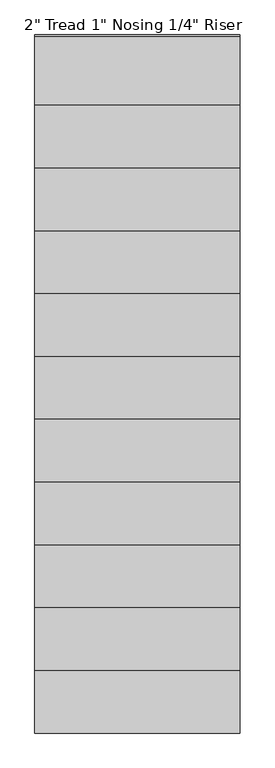
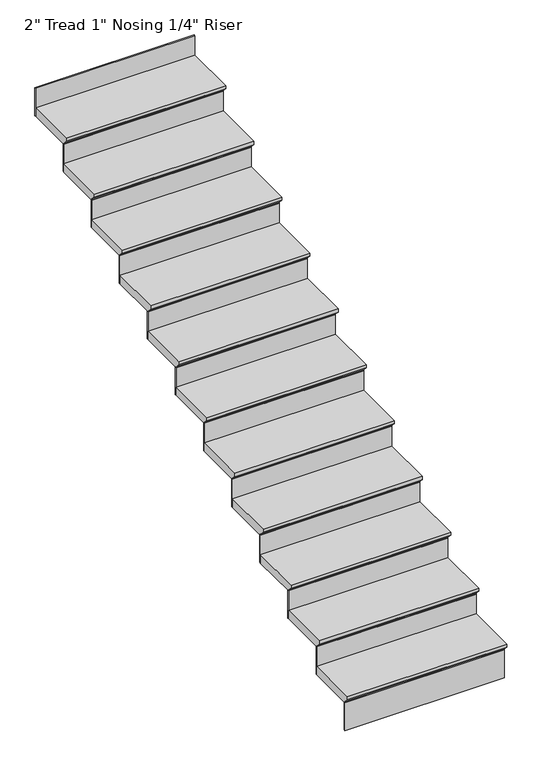
"""IFC4 building model written with IfcOpenShell, lengths in millimetres: stair flight geometry."""

from ifc_helpers import new_model, si_unit, frame, origin, place, context, project, spatial, polyline, outline, extrude, source, transform, mapped, element, save


def stair_flight_b0062ef7(model_context):
    return source(origin(), model_context, "Body", "SweptSolid", [
        extrude(outline(polyline([(-11795.059218, 4233.3333333), (-11490.259218, 4233.3333333), (-11490.259218, 4182.5333333), (-11769.659218, 4182.5333333), (-11769.659218, 4188.8833333), (-11795.059218, 4214.2833333), (-11795.059218, 4233.3333333)])), frame((-1903.2563134, 0.0, 0.0), z_axis=(1.0, 0.0, 0.0), x_axis=(0.0, 1.0, 0.0)), (0.0, 0.0, 1.0), 914.4),
        extrude(outline(polyline([(-988.8563134, -11763.309218), (-988.8563134, -11769.659218), (-1903.2563134, -11769.659218), (-1903.2563134, -11763.309218), (-988.8563134, -11763.309218)])), frame((0.0, 0.0, 4013.2), z_axis=(0.0, 0.0, 1.0), x_axis=(1.0, 0.0, 0.0)), (0.0, 0.0, 1.0), 169.3333333),
        extrude(outline(polyline([(-988.8563134, -11483.909218), (-988.8563134, -11490.259218), (-1903.2563134, -11490.259218), (-1903.2563134, -11483.909218), (-988.8563134, -11483.909218)])), frame((0.0, 0.0, 4182.5333333), z_axis=(0.0, 0.0, 1.0), x_axis=(1.0, 0.0, 0.0)), (0.0, 0.0, 1.0), 169.3333333),
        extrude(outline(polyline([(-11515.659218, 4402.6666667), (-11210.859218, 4402.6666667), (-11210.859218, 4351.8666667), (-11490.259218, 4351.8666667), (-11490.259218, 4358.2166667), (-11515.659218, 4383.6166667), (-11515.659218, 4402.6666667)])), frame((-1903.2563134, 0.0, 0.0), z_axis=(1.0, 0.0, 0.0), x_axis=(0.0, 1.0, 0.0)), (0.0, 0.0, 1.0), 914.4),
        extrude(outline(polyline([(-988.8563134, -11204.509218), (-988.8563134, -11210.859218), (-1903.2563134, -11210.859218), (-1903.2563134, -11204.509218), (-988.8563134, -11204.509218)])), frame((0.0, 0.0, 4351.8666667), z_axis=(0.0, 0.0, 1.0), x_axis=(1.0, 0.0, 0.0)), (0.0, 0.0, 1.0), 169.3333333),
        extrude(outline(polyline([(-11236.259218, 4572.0), (-10931.459218, 4572.0), (-10931.459218, 4521.2), (-11210.859218, 4521.2), (-11210.859218, 4527.55), (-11236.259218, 4552.95), (-11236.259218, 4572.0)])), frame((-1903.2563134, 0.0, 0.0), z_axis=(1.0, 0.0, 0.0), x_axis=(0.0, 1.0, 0.0)), (0.0, 0.0, 1.0), 914.4),
        extrude(outline(polyline([(-988.8563134, -10925.109218), (-988.8563134, -10931.459218), (-1903.2563134, -10931.459218), (-1903.2563134, -10925.109218), (-988.8563134, -10925.109218)])), frame((0.0, 0.0, 4521.2), z_axis=(0.0, 0.0, 1.0), x_axis=(1.0, 0.0, 0.0)), (0.0, 0.0, 1.0), 169.3333333),
        extrude(outline(polyline([(-10956.859218, 4741.3333333), (-10652.059218, 4741.3333333), (-10652.059218, 4690.5333333), (-10931.459218, 4690.5333333), (-10931.459218, 4696.8833333), (-10956.859218, 4722.2833333), (-10956.859218, 4741.3333333)])), frame((-1903.2563134, 0.0, 0.0), z_axis=(1.0, 0.0, 0.0), x_axis=(0.0, 1.0, 0.0)), (0.0, 0.0, 1.0), 914.4),
        extrude(outline(polyline([(-988.8563134, -10645.709218), (-988.8563134, -10652.059218), (-1903.2563134, -10652.059218), (-1903.2563134, -10645.709218), (-988.8563134, -10645.709218)])), frame((0.0, 0.0, 4690.5333333), z_axis=(0.0, 0.0, 1.0), x_axis=(1.0, 0.0, 0.0)), (0.0, 0.0, 1.0), 169.3333333),
        extrude(outline(polyline([(-10677.459218, 4910.6666667), (-10372.659218, 4910.6666667), (-10372.659218, 4859.8666667), (-10652.059218, 4859.8666667), (-10652.059218, 4866.2166667), (-10677.459218, 4891.6166667), (-10677.459218, 4910.6666667)])), frame((-1903.2563134, 0.0, 0.0), z_axis=(1.0, 0.0, 0.0), x_axis=(0.0, 1.0, 0.0)), (0.0, 0.0, 1.0), 914.4),
        extrude(outline(polyline([(-988.8563134, -10366.309218), (-988.8563134, -10372.659218), (-1903.2563134, -10372.659218), (-1903.2563134, -10366.309218), (-988.8563134, -10366.309218)])), frame((0.0, 0.0, 4859.8666667), z_axis=(0.0, 0.0, 1.0), x_axis=(1.0, 0.0, 0.0)), (0.0, 0.0, 1.0), 169.3333333),
        extrude(outline(polyline([(-10398.059218, 5080.0), (-10093.259218, 5080.0), (-10093.259218, 5029.2), (-10372.659218, 5029.2), (-10372.659218, 5035.55), (-10398.059218, 5060.95), (-10398.059218, 5080.0)])), frame((-1903.2563134, 0.0, 0.0), z_axis=(1.0, 0.0, 0.0), x_axis=(0.0, 1.0, 0.0)), (0.0, 0.0, 1.0), 914.4),
        extrude(outline(polyline([(-988.8563134, -10086.909218), (-988.8563134, -10093.259218), (-1903.2563134, -10093.259218), (-1903.2563134, -10086.909218), (-988.8563134, -10086.909218)])), frame((0.0, 0.0, 5029.2), z_axis=(0.0, 0.0, 1.0), x_axis=(1.0, 0.0, 0.0)), (0.0, 0.0, 1.0), 169.3333333),
        extrude(outline(polyline([(-10118.659218, 5249.3333333), (-9813.859218, 5249.3333333), (-9813.859218, 5198.5333333), (-10093.259218, 5198.5333333), (-10093.259218, 5204.8833333), (-10118.659218, 5230.2833333), (-10118.659218, 5249.3333333)])), frame((-1903.2563134, 0.0, 0.0), z_axis=(1.0, 0.0, 0.0), x_axis=(0.0, 1.0, 0.0)), (0.0, 0.0, 1.0), 914.4),
        extrude(outline(polyline([(-988.8563134, -9807.509218), (-988.8563134, -9813.859218), (-1903.2563134, -9813.859218), (-1903.2563134, -9807.509218), (-988.8563134, -9807.509218)])), frame((0.0, 0.0, 5198.5333333), z_axis=(0.0, 0.0, 1.0), x_axis=(1.0, 0.0, 0.0)), (0.0, 0.0, 1.0), 169.3333333),
        extrude(outline(polyline([(-9839.259218, 5418.6666667), (-9534.459218, 5418.6666667), (-9534.459218, 5367.8666667), (-9813.859218, 5367.8666667), (-9813.859218, 5374.2166667), (-9839.259218, 5399.6166667), (-9839.259218, 5418.6666667)])), frame((-1903.2563134, 0.0, 0.0), z_axis=(1.0, 0.0, 0.0), x_axis=(0.0, 1.0, 0.0)), (0.0, 0.0, 1.0), 914.4),
        extrude(outline(polyline([(-988.8563134, -9528.109218), (-988.8563134, -9534.459218), (-1903.2563134, -9534.459218), (-1903.2563134, -9528.109218), (-988.8563134, -9528.109218)])), frame((0.0, 0.0, 5367.8666667), z_axis=(0.0, 0.0, 1.0), x_axis=(1.0, 0.0, 0.0)), (0.0, 0.0, 1.0), 169.3333333),
        extrude(outline(polyline([(-9559.859218, 5588.0), (-9255.059218, 5588.0), (-9255.059218, 5537.2), (-9534.459218, 5537.2), (-9534.459218, 5543.55), (-9559.859218, 5568.95), (-9559.859218, 5588.0)])), frame((-1903.2563134, 0.0, 0.0), z_axis=(1.0, 0.0, 0.0), x_axis=(0.0, 1.0, 0.0)), (0.0, 0.0, 1.0), 914.4),
        extrude(outline(polyline([(-988.8563134, -9248.709218), (-988.8563134, -9255.059218), (-1903.2563134, -9255.059218), (-1903.2563134, -9248.709218), (-988.8563134, -9248.709218)])), frame((0.0, 0.0, 5537.2), z_axis=(0.0, 0.0, 1.0), x_axis=(1.0, 0.0, 0.0)), (0.0, 0.0, 1.0), 169.3333333),
        extrude(outline(polyline([(-9280.459218, 5757.3333333), (-8975.659218, 5757.3333333), (-8975.659218, 5706.5333333), (-9255.059218, 5706.5333333), (-9255.059218, 5712.8833333), (-9280.459218, 5738.2833333), (-9280.459218, 5757.3333333)])), frame((-1903.2563134, 0.0, 0.0), z_axis=(1.0, 0.0, 0.0), x_axis=(0.0, 1.0, 0.0)), (0.0, 0.0, 1.0), 914.4),
        extrude(outline(polyline([(-988.8563134, -8969.309218), (-988.8563134, -8975.659218), (-1903.2563134, -8975.659218), (-1903.2563134, -8969.309218), (-988.8563134, -8969.309218)])), frame((0.0, 0.0, 5706.5333333), z_axis=(0.0, 0.0, 1.0), x_axis=(1.0, 0.0, 0.0)), (0.0, 0.0, 1.0), 169.3333333),
        extrude(outline(polyline([(-988.8563134, -8689.909218), (-988.8563134, -8696.259218), (-1903.2563134, -8696.259218), (-1903.2563134, -8689.909218), (-988.8563134, -8689.909218)])), frame((0.0, 0.0, 5875.8666667), z_axis=(0.0, 0.0, 1.0), x_axis=(1.0, 0.0, 0.0)), (0.0, 0.0, 1.0), 169.3333333),
        extrude(outline(polyline([(-9001.059218, 5926.6666667), (-8696.259218, 5926.6666667), (-8696.259218, 5875.8666667), (-8975.659218, 5875.8666667), (-8975.659218, 5882.2166667), (-9001.059218, 5907.6166667), (-9001.059218, 5926.6666667)])), frame((-1903.2563134, 0.0, 0.0), z_axis=(1.0, 0.0, 0.0), x_axis=(0.0, 1.0, 0.0)), (0.0, 0.0, 1.0), 914.4),
    ])


if __name__ == "__main__":
    model = new_model("IFC4")
    model_context = context("Model", 3, world=origin())
    ifc_project = project(units=[si_unit("LENGTHUNIT", "METRE", prefix="MILLI")], contexts=[model_context])
    site = spatial("IfcSite", under=ifc_project)
    building = spatial("IfcBuilding", under=site)
    placement = place(None, origin())
    stair_flight_shape = stair_flight_b0062ef7(model_context)
    element("IfcStairFlight", 1, ObjectType="2\" Tread 1\" Nosing 1/4\" Riser", at=placement, inside=building, context=model_context, shape_type="MappedRepresentation", body=[
        mapped(stair_flight_shape, transform((0.0, 0.0, 0.0), x_axis=(1.0, 0.0, 0.0), y_axis=(0.0, 1.0, 0.0), z_axis=(0.0, 0.0, 1.0))),
    ])
    save(model, "model.ifc")
